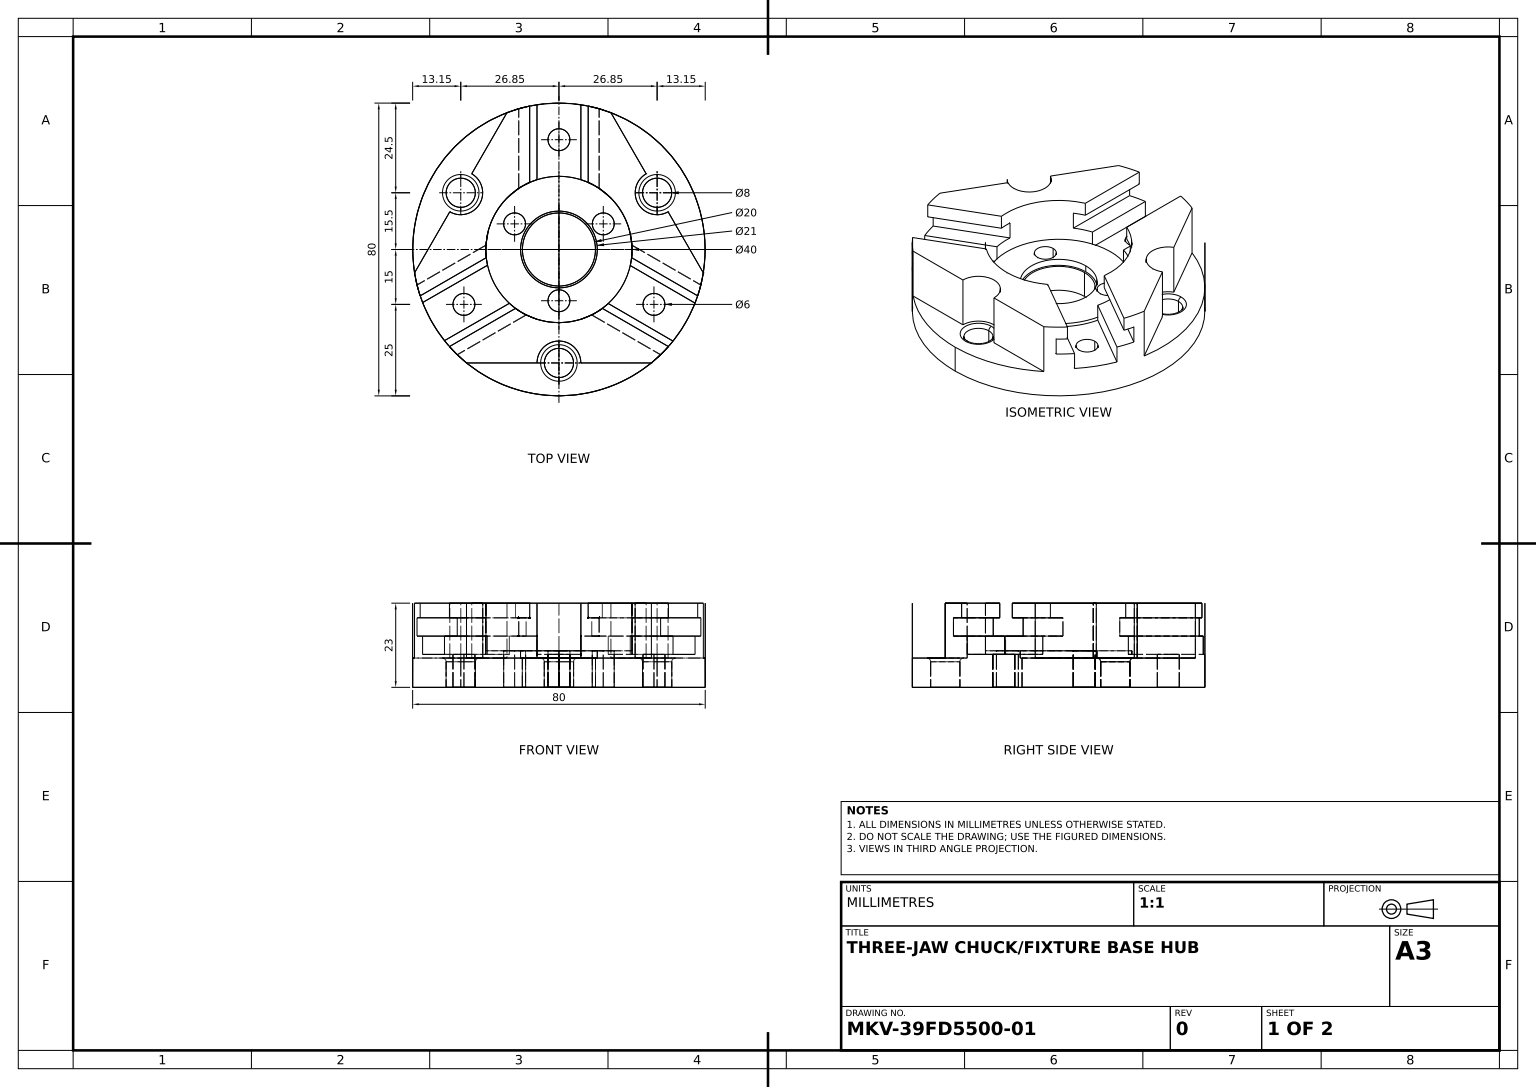
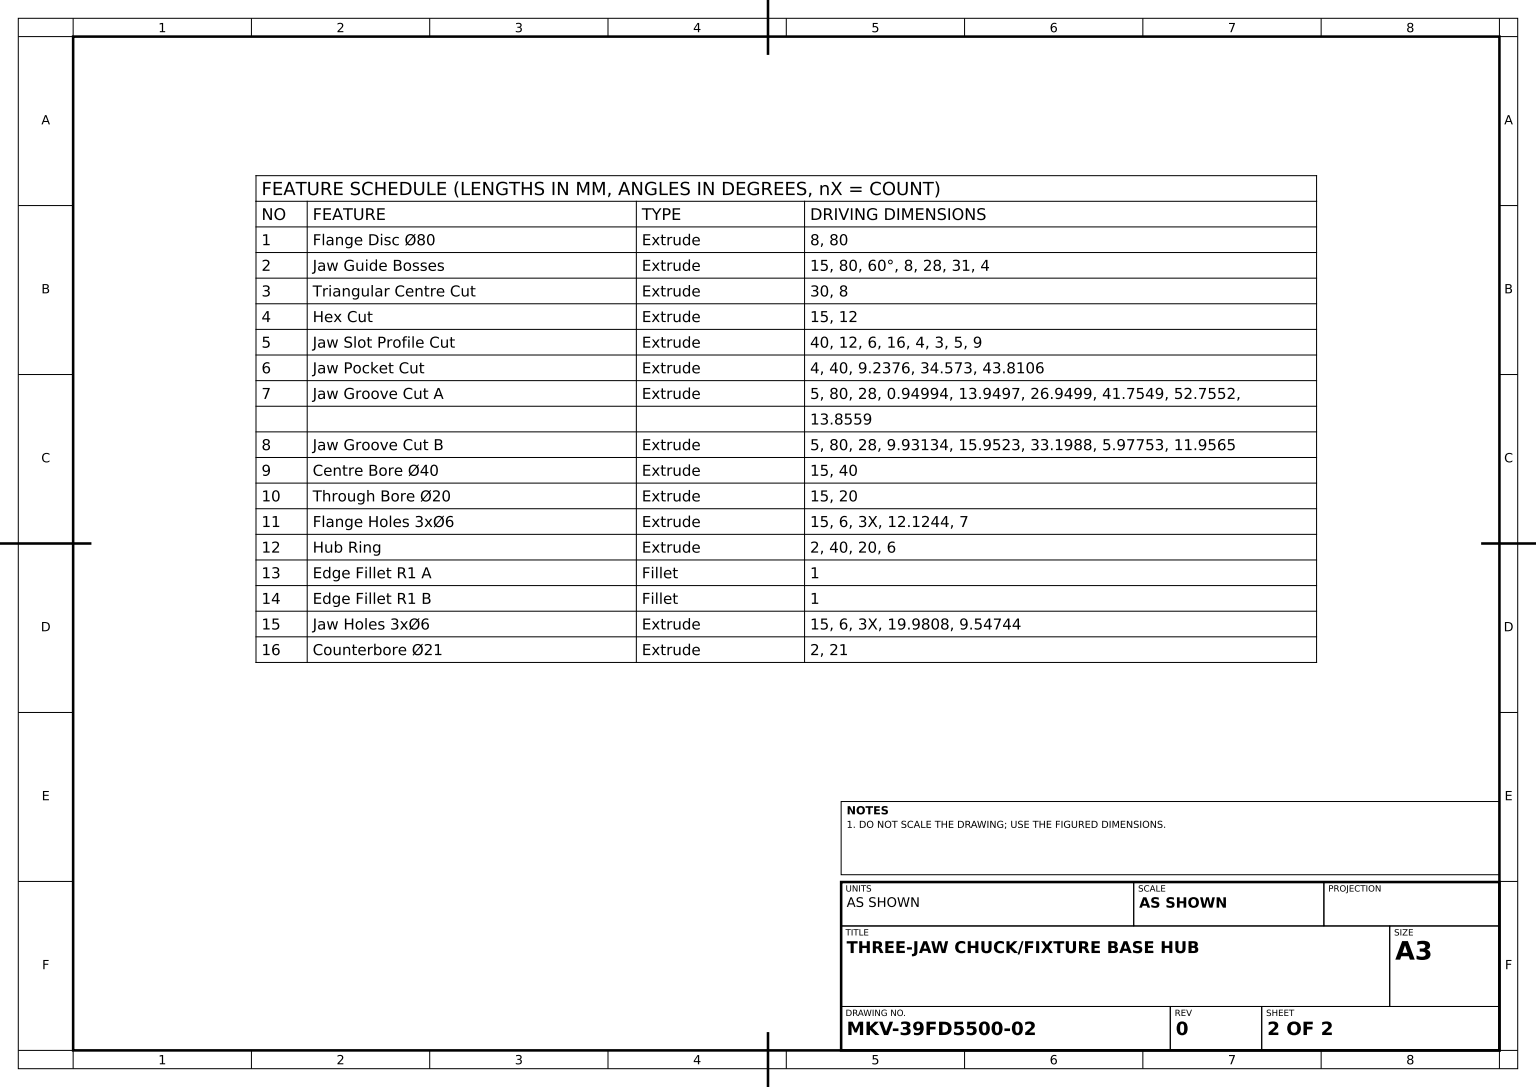
from build123d import *
from build123d.topology import SkipClean

# Parameters (mm, degrees)
FLANGE_DISC_SKETCH_R           = 40
FLANGE_DISC_80_DEPTH           = 8
JAW_GUIDE_BOSSES_SKETCH_R      = 14
JAW_GUIDE_BOSSES_DEPTH         = 15
TRIANGULAR_START               = -30
TRIANGULAR_CENTRE_CUT_SKETCH_R = 4
TRIANGULAR_CENTRE_CUT_DEPTH    = 30
HEX_CUT_DEPTH                  = 15
JAW_SLOT_PROFILE_CUT_DEPTH     = 40
JAW_START                      = -4
JAW_POCKET_CUT_DEPTH           = 4
JAW_START_2                    = -5
JAW_GROOVE_CUT_A_DEPTH         = 5
JAW_GROOVE_CUT_B_DEPTH         = 5
CENTRE_BORE_SKETCH_R           = 20
CENTRE_BORE_40_DEPTH           = 15
THROUGH_BORE_SKETCH_R          = 10
THROUGH_BORE_20_DEPTH          = 15
FLANGE_HOLES_SKETCH_R          = 3
FLANGE_HOLES_3X_6_DEPTH        = 15
HUB_START                      = 2
HUB_RING_SKETCH_R              = 20
HUB_RING_SKETCH_R_2            = 10
HUB_RING_SKETCH_R_3            = 3
HUB_RING_DEPTH                 = 2
EDGE_FILLET_R1_A_R             = 1
EDGE_FILLET_R1_B_R             = 1
JAW_HOLES_SKETCH_R             = 3
JAW_HOLES_3X_6_DEPTH           = 15
COUNTERBORE_SKETCH_R           = 10.5
COUNTERBORE_21_DEPTH           = 2


with BuildPart() as part:
    # Flange Disc Sketch → Flange Disc Ø80 (new body)
    with BuildSketch(Plane(origin=(0, 0, 0), x_dir=(1, 0, 0), z_dir=(0, 1, 0))):
        with Locations(Location((0, 0, 0), (0, 0, 270))):
            Circle(FLANGE_DISC_SKETCH_R)
    extrude(amount=FLANGE_DISC_80_DEPTH)

    # Jaw Guide Bosses Sketch → Jaw Guide Bosses (add)
    with BuildSketch(Plane(origin=(0, 8, 0), x_dir=(1, 0, 0), z_dir=(0, 1, 0))):
        with BuildLine():
            ThreePointArc((-22.846787517, 15.5), (-24.846787517, 12.035898385), (-28.846787517, 12.035898385))
            Line((-28.846787517, 12.035898385), (-39.486012177, -6.391779279))
            ThreePointArc((-39.486012177, -6.391779279), (-34.641016151, -20), (-25.27844932, -31))
            Line((-25.27844932, -31), (-4, -31))
            ThreePointArc((-4, -31), (0, -27), (4, -31))
            Line((4, -31), (25.27844932, -31))
            ThreePointArc((25.27844932, -31), (34.641016151, -20), (39.486012177, -6.391779279))
            Line((39.486012177, -6.391779279), (28.846787517, 12.035898385))
            ThreePointArc((28.846787517, 12.035898385), (23.382685902, 13.5), (24.846787517, 18.964101615))
            Line((24.846787517, 18.964101615), (14.207562858, 37.391779279))
            ThreePointArc((14.207562858, 37.391779279), (0, 40), (-14.207562858, 37.391779279))
            Line((-14.207562858, 37.391779279), (-24.846787517, 18.964101615))
            ThreePointArc((-24.846787517, 18.964101615), (-23.382685902, 17.5), (-22.846787517, 15.5))
        make_face()
        with Locations(Location((0, 0, 0), (0, 0, 270))):
            Circle(JAW_GUIDE_BOSSES_SKETCH_R, mode=Mode.SUBTRACT)
    extrude(amount=JAW_GUIDE_BOSSES_DEPTH)

    # Triangular Centre Cut Sketch → Triangular Centre Cut (cut)
    with SkipClean():  # the faces are left unmerged after this step: merging them gives an invalid solid
        with BuildSketch(Plane(origin=(0, 23, 0), x_dir=(1, 0, 0), z_dir=(0, 1, 0)).offset(TRIANGULAR_START)):
            with Locations(Location((-26.846787517, 15.5, 0), (0, 0, 60))):
                Circle(TRIANGULAR_CENTRE_CUT_SKETCH_R)
            with Locations(Location((26.846787517, 15.5, 0), (0, 0, 120))):
                Circle(TRIANGULAR_CENTRE_CUT_SKETCH_R)
            with Locations((0, -31)):
                Circle(TRIANGULAR_CENTRE_CUT_SKETCH_R)
        extrude(amount=TRIANGULAR_CENTRE_CUT_DEPTH, mode=Mode.SUBTRACT)

    # Hex Cut Sketch → Hex Cut (cut)
    with BuildSketch(Plane(origin=(0, 23, 0), x_dir=(1, 0, 0), z_dir=(0, 1, 0))):
        with BuildLine():
            Line((-29.846787517, 10.303847577), (-23.846787517, 20.696152423))
            ThreePointArc((-23.846787517, 20.696152423), (-21.650635095, 12.5), (-29.846787517, 10.303847577))
        make_face()
        with BuildLine():
            Line((23.846787517, 20.696152423), (29.846787517, 10.303847577))
            ThreePointArc((29.846787517, 10.303847577), (21.650635095, 12.5), (23.846787517, 20.696152423))
        make_face()
        with BuildLine():
            Line((-6, -31), (6, -31))
            ThreePointArc((6, -31), (0, -25), (-6, -31))
        make_face()
    extrude(amount=-HEX_CUT_DEPTH, mode=Mode.SUBTRACT)

    # Jaw Slot Profile Sketch → Jaw Slot Profile Cut (cut)
    with BuildSketch(Plane.XY.offset(-40)):
        Polygon((8, 23), (-8, 23), (-8, 19), (-11, 19), (-11, 14), (-6, 14), (-6, 9), (6, 9), (6, 14), (11, 14), (11, 19), (8, 19), align=None)
    extrude(amount=JAW_SLOT_PROFILE_CUT_DEPTH, mode=Mode.SUBTRACT)

    # Jaw Pocket Sketch → Jaw Pocket Cut (cut)
    with BuildSketch(Plane(origin=(0, 23, 0), x_dir=(1, 0, 0), z_dir=(0, 1, 0)).offset(JAW_START)):
        with BuildLine():
            Line((0, 9.237604307), (37.941125497, -12.667714712))
            ThreePointArc((37.941125497, -12.667714712), (34.641016151, -20), (29.941125497, -26.524121173))
            Line((29.941125497, -26.524121173), (0, -9.237604307))
            Line((0, -9.237604307), (-29.941125497, -26.524121173))
            ThreePointArc((-29.941125497, -26.524121173), (-34.641016151, -20), (-37.941125497, -12.667714712))
            Line((-37.941125497, -12.667714712), (0, 9.237604307))
        make_face()
    extrude(amount=JAW_POCKET_CUT_DEPTH, mode=Mode.SUBTRACT)

    # Jaw Groove Sketch A → Jaw Groove Cut A (cut)
    with BuildSketch(Plane(origin=(0, 19, 0), x_dir=(1, 0, 0), z_dir=(0, 1, 0)).offset(JAW_START_2)):
        with BuildLine():
            Line((-27.805770218, -28.754810773), (-2.000176006, -13.856381055))
            ThreePointArc((-2.000176006, -13.856381055), (-4.018838324, -13.410776955), (-5.949874371, -12.672765877))
            Line((-5.949874371, -12.672765877), (-29.941125497, -26.524121173))
            ThreePointArc((-29.941125497, -26.524121173), (-28.894982007, -27.660079805), (-27.805770218, -28.754810773))
        make_face()
        with BuildLine():
            Line((-37.941125497, -12.667714712), (-13.949874371, 1.183640584))
            ThreePointArc((-13.949874371, 1.183640584), (-13.623451724, 3.225145443), (-12.999933997, 5.196317551))
            Line((-12.999933997, 5.196317551), (-38.805528208, -9.702112168))
            ThreePointArc((-38.805528208, -9.702112168), (-38.401964967, -11.19326077), (-37.941125497, -12.667714712))
        make_face()
        with BuildLine():
            ThreePointArc((-5.949874371, -12.672765877), (-12.124355653, -7), (-13.949874371, 1.183640584))
            Line((-13.949874371, 1.183640584), (-37.941125497, -12.667714712))
            ThreePointArc((-37.941125497, -12.667714712), (-34.641016151, -20), (-29.941125497, -26.524121173))
            Line((-29.941125497, -26.524121173), (-5.949874371, -12.672765877))
        make_face()
        with BuildLine():
            Line((38.805281719, -9.703097994), (13.000066001, 5.195987294))
            ThreePointArc((13.000066001, 5.195987294), (12.124266737, -7.000154005), (1.999823994, -13.856431864))
            Line((1.999823994, -13.856431864), (27.805039711, -28.755517151))
            ThreePointArc((27.805039711, -28.755517151), (34.640762105, -20.000440015), (38.805281719, -9.703097994))
        make_face()
    extrude(amount=JAW_GROOVE_CUT_A_DEPTH, mode=Mode.SUBTRACT)

    # Jaw Groove Sketch B → Jaw Groove Cut B (cut)
    with BuildSketch(Plane(origin=(0, 14, 0), x_dir=(1, 0, 0), z_dir=(0, 1, 0)).offset(JAW_START_2)):
        with BuildLine():
            Line((13.952143608, -1.156584943), (37.219568724, -14.652771205))
            ThreePointArc((37.219568724, -14.652771205), (34.600550719, -20.069925011), (31.198591221, -25.03293642))
            Line((31.198591221, -25.03293642), (7.931166105, -11.536750158))
            ThreePointArc((7.931166105, -11.536750158), (12.110192752, -7.024473754), (13.952143608, -1.156584943))
        make_face()
        with BuildLine():
            Line((-13.956701767, -1.10021625), (-37.278454482, -14.50230435))
            ThreePointArc((-37.278454482, -14.50230435), (-34.681340271, -19.929993402), (-31.299456461, -24.906706431))
            Line((-31.299456461, -24.906706431), (-7.977703746, -11.504618331))
            ThreePointArc((-7.977703746, -11.504618331), (-12.138469095, -6.975497691), (-13.956701767, -1.10021625))
        make_face()
    extrude(amount=JAW_GROOVE_CUT_B_DEPTH, mode=Mode.SUBTRACT)

    # Centre Bore Sketch → Centre Bore Ø40 (cut)
    with BuildSketch(Plane(origin=(0, 23, 0), x_dir=(1, 0, 0), z_dir=(0, 1, 0))):
        with Locations(Location((0, 0, 0), (0, 0, 270))):
            Circle(CENTRE_BORE_SKETCH_R)
    extrude(amount=-CENTRE_BORE_40_DEPTH, mode=Mode.SUBTRACT)

    # Through Bore Sketch → Through Bore Ø20 (cut)
    with BuildSketch(Plane(origin=(0, 8, 0), x_dir=(1, 0, 0), z_dir=(0, 1, 0))):
        with Locations(Location((0, 0, 0), (0, 0, 270))):
            Circle(THROUGH_BORE_SKETCH_R)
    extrude(amount=-THROUGH_BORE_20_DEPTH, mode=Mode.SUBTRACT)

    # Flange Holes Sketch → Flange Holes 3xØ6 (cut)
    with BuildSketch(Plane(origin=(0, 8, 0), x_dir=(1, 0, 0), z_dir=(0, 1, 0))):
        with Locations(Location((0, -14, 0), (0, 0, 270))):
            Circle(FLANGE_HOLES_SKETCH_R)
        with Locations(Location((-12.124355653, 7, 0), (0, 0, 270))):
            Circle(FLANGE_HOLES_SKETCH_R)
        with Locations(Location((12.124355653, 7, 0), (0, 0, 270))):
            Circle(FLANGE_HOLES_SKETCH_R)
    extrude(amount=-FLANGE_HOLES_3X_6_DEPTH, mode=Mode.SUBTRACT)

    # Hub Ring Sketch → Hub Ring (add)
    with BuildSketch(Plane(origin=(0, 8, 0), x_dir=(1, 0, 0), z_dir=(0, 1, 0)).offset(HUB_START)):
        Circle(HUB_RING_SKETCH_R)
        with Locations(Location((0, 0, 0), (0, 0, 270))):
            Circle(HUB_RING_SKETCH_R_2, mode=Mode.SUBTRACT)
        with Locations(Location((-12.124355653, 7, 0), (0, 0, 270))):
            Circle(HUB_RING_SKETCH_R_3, mode=Mode.SUBTRACT)
        with Locations(Location((12.124355653, 7, 0), (0, 0, 270))):
            Circle(HUB_RING_SKETCH_R_3, mode=Mode.SUBTRACT)
        with Locations(Location((0, -14, 0), (0, 0, 270))):
            Circle(HUB_RING_SKETCH_R_3, mode=Mode.SUBTRACT)
    extrude(amount=-HUB_RING_DEPTH)

    # Edge Fillet R1 A
    edge_fillet_r1_a_edges = [part.edges().sort_by_distance(p)[0] for p in [
        (28.846787517, 8, -12.035898385),
    ]]
    fillet(edge_fillet_r1_a_edges, radius=EDGE_FILLET_R1_A_R)

    # Edge Fillet R1 B
    edge_fillet_r1_b_edges = [part.edges().sort_by_distance(p)[0] for p in [
        (-28.846787517, 8, -12.035898385),
        (-4, 8, 31),
    ]]
    fillet(edge_fillet_r1_b_edges, radius=EDGE_FILLET_R1_B_R)

    # Jaw Holes Sketch → Jaw Holes 3xØ6 (cut)
    with BuildSketch(Plane(origin=(0, 9, 0), x_dir=(1, 0, 0), z_dir=(0, 1, 0))):
        with Locations(Location((0, 30, 0), (0, 0, 270))):
            Circle(JAW_HOLES_SKETCH_R)
        with Locations(Location((25.980762114, -15, 0), (0, 0, 270))):
            Circle(JAW_HOLES_SKETCH_R)
        with Locations(Location((-25.980762114, -15, 0), (0, 0, 270))):
            Circle(JAW_HOLES_SKETCH_R)
    extrude(amount=-JAW_HOLES_3X_6_DEPTH, mode=Mode.SUBTRACT)

    # Counterbore Sketch → Counterbore Ø21 (cut)
    with BuildSketch(Plane(origin=(0, 10, 0), x_dir=(1, 0, 0), z_dir=(0, 1, 0))):
        with Locations(Location((0, 0, 0), (0, 0, 270))):
            Circle(COUNTERBORE_SKETCH_R)
    extrude(amount=-COUNTERBORE_21_DEPTH, mode=Mode.SUBTRACT)


solid = part.part
